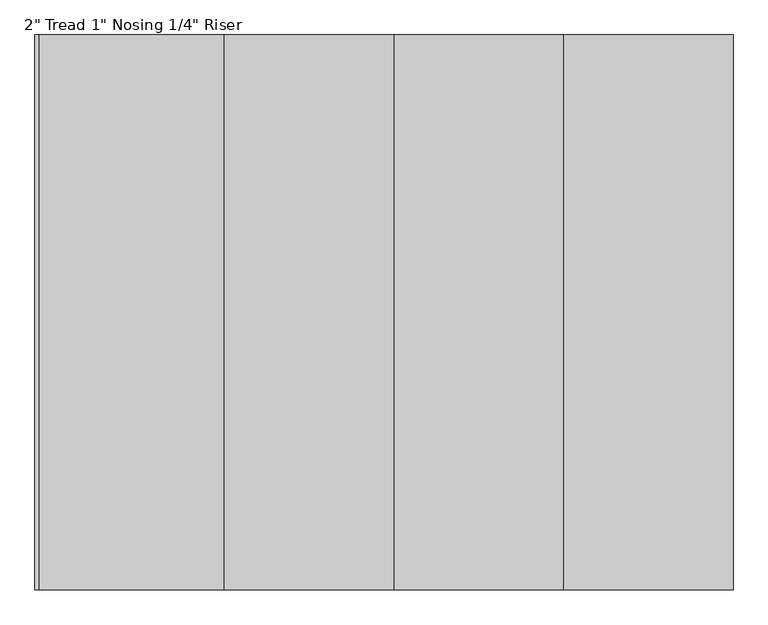
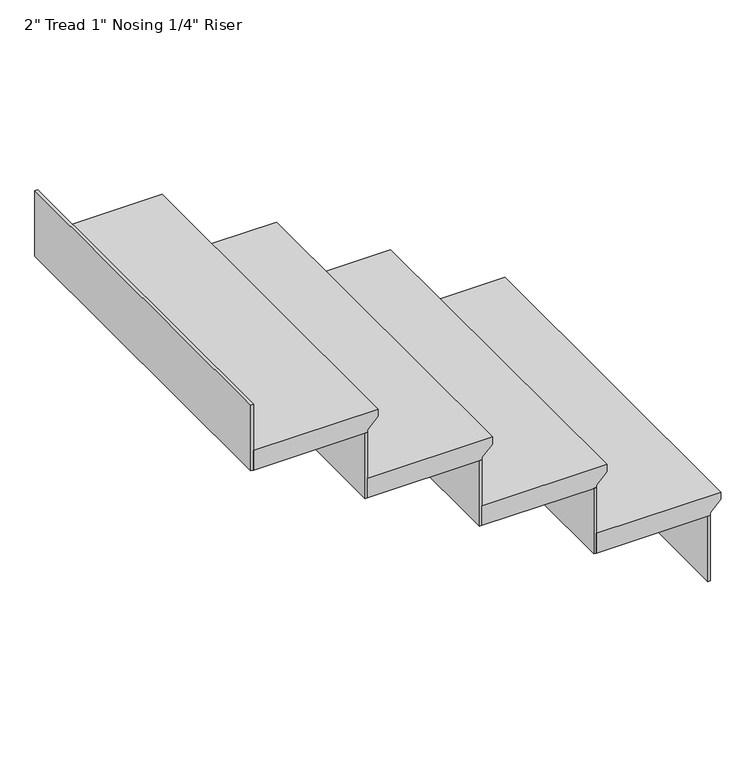
"""IFC4 building model written with IfcOpenShell, lengths in millimetres: stair flight geometry."""

from ifc_helpers import new_model, si_unit, frame, origin, place, context, project, spatial, polyline, outline, extrude, source, transform, mapped, element, save


def stair_flight_f110103f(model_context):
    return source(origin(), model_context, "Body", "SweptSolid", [
        extrude(outline(polyline([(5418.6666667, -803.1608498), (5418.6666667, -1107.9608498), (5367.8666667, -1107.9608498), (5367.8666667, -828.5608498), (5374.2166667, -828.5608498), (5399.6166667, -803.1608498), (5418.6666667, -803.1608498)])), frame((0.0, 1203.1115866, 0.0), z_axis=(0.0, 1.0, 0.0), x_axis=(0.0, 0.0, 1.0)), (0.0, 0.0, 1.0), 914.4),
        extrude(outline(polyline([(-834.9108498, 2117.5115866), (-828.5608498, 2117.5115866), (-828.5608498, 1203.1115866), (-834.9108498, 1203.1115866), (-834.9108498, 2117.5115866)])), frame((0.0, 0.0, 5198.5333333), z_axis=(0.0, 0.0, 1.0), x_axis=(1.0, 0.0, 0.0)), (0.0, 0.0, 1.0), 169.3333333),
        extrude(outline(polyline([(-1114.3108498, 2117.5115866), (-1107.9608498, 2117.5115866), (-1107.9608498, 1203.1115866), (-1114.3108498, 1203.1115866), (-1114.3108498, 2117.5115866)])), frame((0.0, 0.0, 5367.8666667), z_axis=(0.0, 0.0, 1.0), x_axis=(1.0, 0.0, 0.0)), (0.0, 0.0, 1.0), 169.3333333),
        extrude(outline(polyline([(5588.0, -1082.5608498), (5588.0, -1387.3608498), (5537.2, -1387.3608498), (5537.2, -1107.9608498), (5543.55, -1107.9608498), (5568.95, -1082.5608498), (5588.0, -1082.5608498)])), frame((0.0, 1203.1115866, 0.0), z_axis=(0.0, 1.0, 0.0), x_axis=(0.0, 0.0, 1.0)), (0.0, 0.0, 1.0), 914.4),
        extrude(outline(polyline([(-1393.7108498, 2117.5115866), (-1387.3608498, 2117.5115866), (-1387.3608498, 1203.1115866), (-1393.7108498, 1203.1115866), (-1393.7108498, 2117.5115866)])), frame((0.0, 0.0, 5537.2), z_axis=(0.0, 0.0, 1.0), x_axis=(1.0, 0.0, 0.0)), (0.0, 0.0, 1.0), 169.3333333),
        extrude(outline(polyline([(5757.3333333, -1361.9608498), (5757.3333333, -1666.7608498), (5706.5333333, -1666.7608498), (5706.5333333, -1387.3608498), (5712.8833333, -1387.3608498), (5738.2833333, -1361.9608498), (5757.3333333, -1361.9608498)])), frame((0.0, 1203.1115866, 0.0), z_axis=(0.0, 1.0, 0.0), x_axis=(0.0, 0.0, 1.0)), (0.0, 0.0, 1.0), 914.4),
        extrude(outline(polyline([(-1673.1108498, 2117.5115866), (-1666.7608498, 2117.5115866), (-1666.7608498, 1203.1115866), (-1673.1108498, 1203.1115866), (-1673.1108498, 2117.5115866)])), frame((0.0, 0.0, 5706.5333333), z_axis=(0.0, 0.0, 1.0), x_axis=(1.0, 0.0, 0.0)), (0.0, 0.0, 1.0), 169.3333333),
        extrude(outline(polyline([(-1952.5108498, 2117.5115866), (-1946.1608498, 2117.5115866), (-1946.1608498, 1203.1115866), (-1952.5108498, 1203.1115866), (-1952.5108498, 2117.5115866)])), frame((0.0, 0.0, 5875.8666667), z_axis=(0.0, 0.0, 1.0), x_axis=(1.0, 0.0, 0.0)), (0.0, 0.0, 1.0), 169.3333333),
        extrude(outline(polyline([(5926.6666667, -1641.3608498), (5926.6666667, -1946.1608498), (5875.8666667, -1946.1608498), (5875.8666667, -1666.7608498), (5882.2166667, -1666.7608498), (5907.6166667, -1641.3608498), (5926.6666667, -1641.3608498)])), frame((0.0, 1203.1115866, 0.0), z_axis=(0.0, 1.0, 0.0), x_axis=(0.0, 0.0, 1.0)), (0.0, 0.0, 1.0), 914.4),
    ])


if __name__ == "__main__":
    model = new_model("IFC4")
    model_context = context("Model", 3, world=origin())
    ifc_project = project(units=[si_unit("LENGTHUNIT", "METRE", prefix="MILLI")], contexts=[model_context])
    site = spatial("IfcSite", under=ifc_project)
    building = spatial("IfcBuilding", under=site)
    placement = place(None, origin())
    stair_flight_shape = stair_flight_f110103f(model_context)
    element("IfcStairFlight", 1, ObjectType="2\" Tread 1\" Nosing 1/4\" Riser", at=placement, inside=building, context=model_context, shape_type="MappedRepresentation", body=[
        mapped(stair_flight_shape, transform((0.0, 0.0, 0.0), x_axis=(1.0, 0.0, 0.0), y_axis=(0.0, 1.0, 0.0), z_axis=(0.0, 0.0, 1.0))),
    ])
    save(model, "model.ifc")
